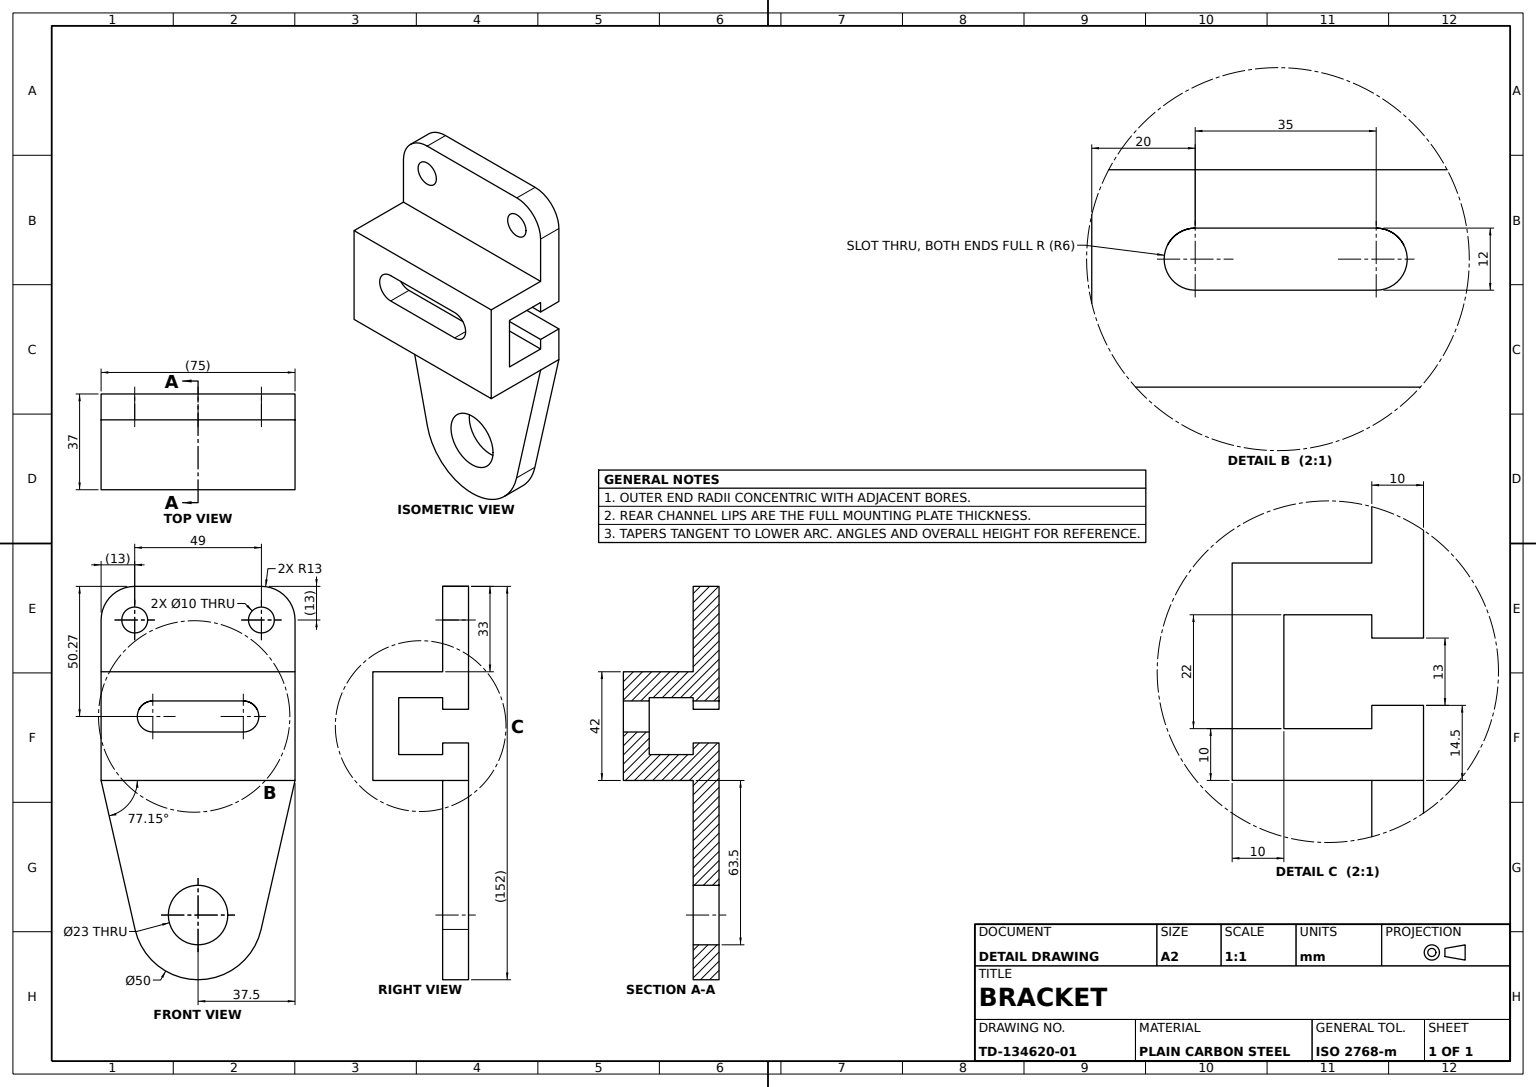
SolidWorks part; units mm, degrees
material "Plain Carbon Steel"
ref_plane "Front Plane" through (0, 0, 0) normal (0, 0, 1) x (1, 0, 0)
ref_plane "Top Plane" through (0, 0, 0) normal (0, 1, 0) x (1, 0, 0)
ref_plane "Right Plane" through (0, 0, 0) normal (1, 0, 0) x (0, 0, -1)
sketch "Bracket Profile Sketch" plane through (0, 0, 0) normal (0, 0, 1) x (1, 0, 0)
  line L0 (0, 103.0058) -> (0, -108.6243) construction
  line L1 (-24.5, 63.5) -> (24.5, 63.5)
  line L2 (-37.5, 50.5) -> (-37.5, -11.5)
  line L4 (37.5, 50.5) -> (37.5, -11.5)
  line L5 (-37.5, 63.5) -> (37.5, -63.5) construction
  line L6 (-37.5, -63.5) -> (37.5, 63.5) construction
  line L7 (-17.5, 13.2268) -> (17.5, 13.2268) construction
  line L8 (-37.5, -11.5) -> (-24.3743, -69.0584)
  line L9 (24.3743, -69.0584) -> (37.5, -11.5)
  line L10 (-37.5, -11.5) -> (37.5, -11.5) construction
  line L11 (-17.5, 19.2268) -> (17.5, 19.2268)
  line L12 (-17.5, 7.2268) -> (17.5, 7.2268)
  circle A0 centre (0, -63.5) radius 11.5
  arc A1 (-24.3743, -69.0584) -> (24.3743, -69.0584) centre (0, -63.5) ccw
  arc A2 (24.5, 63.5) -> (37.5, 50.5) centre (24.5, 50.5) cw
  arc A3 (-24.5, 63.5) -> (-37.5, 50.5) centre (-24.5, 50.5) ccw
  circle A4 centre (-24.5, 50.5) radius 5
  circle A5 centre (24.5, 50.5) radius 5
  arc A6 (-17.5, 19.2268) -> (-17.5, 7.2268) centre (-17.5, 13.2268) ccw
  arc A7 (17.5, 7.2268) -> (17.5, 19.2268) centre (17.5, 13.2268) ccw
  point P0 (0, 0)
  point P25 (0, 13.2268)
  dimension "D3" = 23
  dimension "D4" = 50
  dimension "D6" = 6
  dimension "D2" = 13
  dimension "D5" = 10
  dimension "D1" = 75
  dimension "D7" = 35
  dimension "D8" = 13.1257
  dimension "D9" = 50.2732
  dimension "D10" = 63.5
extrude "Bracket Body" add sketch "Bracket Profile Sketch" along normal blind 37 contours L1 A3 L2 L8 A1 L9 L4 A2 A7 L12 A6 L11 A5 A4 A0
sketch "Slot and Channel Sketch" plane through (0, 0, 0) normal (1, 0, 0) x (0, 0, -1)
  line L0 (0, -69.0584) -> (0, -11.5) construction
  line L1 (-37, 30.5) -> (0, 30.5)
  line L2 (-37, 30.5) -> (-37, -11.5)
  line L3 (-37, -11.5) -> (0, -11.5)
  line L4 (0, 30.5) -> (0, -11.5)
  line L5 (-37, 30.5) -> (0, -11.5) construction
  line L6 (-37, -11.5) -> (0, 30.5) construction
  line L7 (-37, 63.5) -> (0, 63.5) construction
  line L8 (-10, 16) -> (0, 16)
  line L13 (-29.9458, 22.4926) -> (-7.0542, -3.4926) construction
  line L14 (-29.9458, -3.4926) -> (-7.0542, 22.4926) construction
  line L15 (-10, 3) -> (0, 3)
  line L16 (-18.5, 9.5) -> (9.954, 9.5) construction
  line L17 (-10, 3) -> (-10, -1.5)
  line L18 (-27, 20.5) -> (-10, 20.5)
  line L19 (-10, 20.5) -> (-10, 16)
  line L20 (-27, -1.5) -> (-10, -1.5)
  line L21 (-27, 20.5) -> (-27, -1.5)
  line L22 (-10, 30.5) -> (-10, 63.5)
  line L23 (-10, 20.5) -> (-10, -1.5) construction
  line L24 (-10, 63.5) -> (-37, 63.5)
  line L25 (-37, 63.5) -> (-37, 30.5)
  line L27 (-37, -88.5) -> (-10, -88.5)
  line L28 (-37, -88.5) -> (0, -88.5) construction
  line L29 (-10, -88.5) -> (-10, -11.5)
  line L30 (-37, -88.5) -> (-37, -11.5)
  line L31 (-10, 30.5) -> (-37, 30.5)
  line L32 (-37, 63.5) -> (-37, 30.5)
  point P0 (-18.5, 9.5)
  point P9 (-18.5, 9.5)
  dimension "D1" = 42
  dimension "D2" = 33
  dimension "D3" = 37
  dimension "D5" = 13
  dimension "D6" = 6.5
  dimension "D7" = 10
  dimension "D4" = 10
extrude "Slot and Channel Cut" cut sketch "Slot and Channel Sketch" against normal through all both and the other way through all contours L24 L25 L1 L22 | L18 L21 L20 L17 L15 L4 L8 L19 | L30 L27 L29 L3
